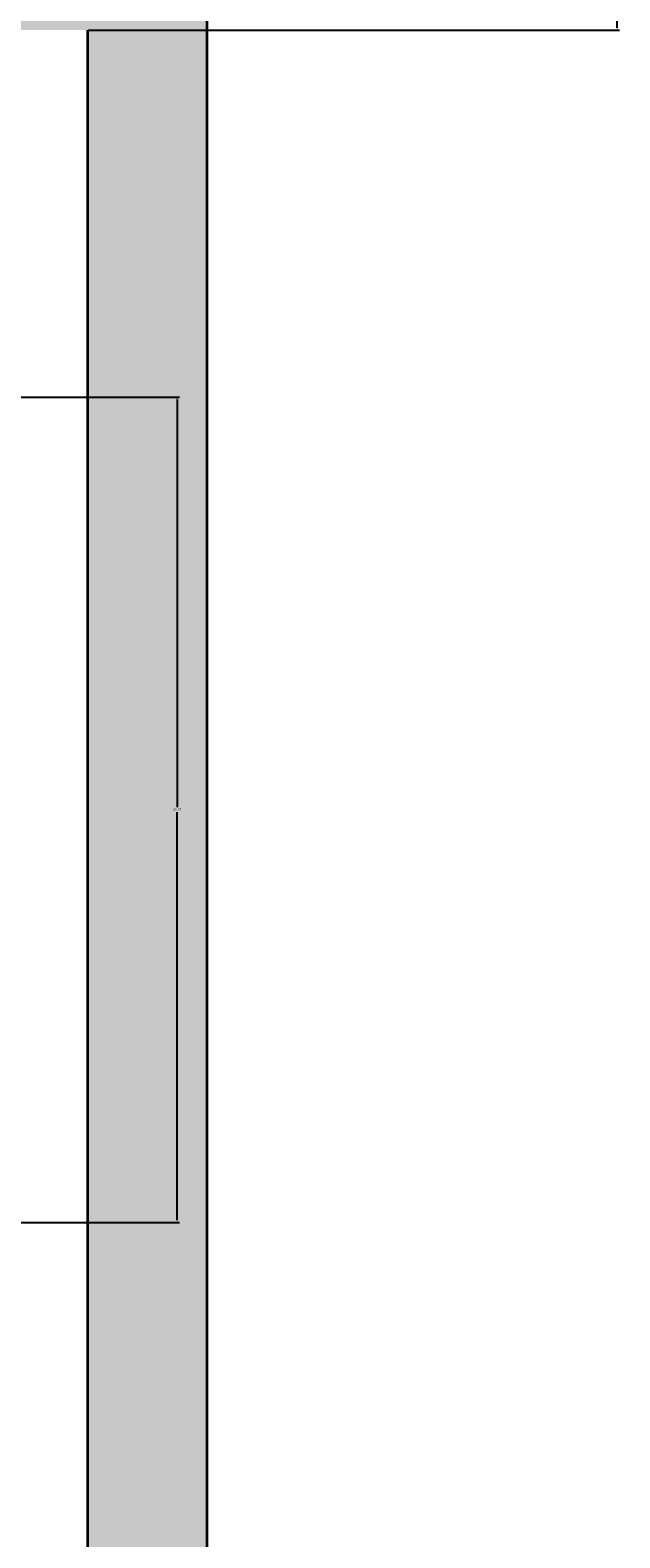
# Model space of a CAD drawing. Units: inches. Extents: x -30 to 437, y -29 to 647.
# Tile 13 of 15: x 392 to 437, y 321 to 435. Entities that reach past the tile are written whole.
import ezdxf

# ---------------------------------------------------------------- set-up
doc = ezdxf.new("R2010")
doc.units = ezdxf.units.IN
doc.header["$MEASUREMENT"] = 0
doc.layers.add('A-ANNO-DIMS', color=2, linetype='Continuous', lineweight=18)
doc.layers.add('A-WALL', color=7, linetype='Continuous', lineweight=35)
doc.layers.add('A-WALL-PATT', color=251, linetype='Continuous', lineweight=13, true_color=0x636466)
doc.styles.get("Standard").update_dxf_attribs({"font": 'arial.ttf'})
doc.dimstyles.get("Standard").update_dxf_attribs({"dimtxt": 0.18, "dimasz": 0.18, "dimexe": 0.18, "dimexo": 0.0625, "dimgap": 0.09, "dimtad": 0, "dimtih": 1, "dimtoh": 1, "dimdec": 4, "dimzin": 0, "dimdsep": 46, "dimtxsty": 'Standard', "dimcen": 0.09, "dimadec": 0, "dimazin": 0, "dimtfac": 1, "dimtdec": 4, "dimtofl": 0, "dimtmove": 0, "dimatfit": 3, "dimfxl": 1, "dimtolj": 1, "dimtzin": 0, "dimarcsym": 0})

# ---------------------------------------------------------------- blocks, each defined once
blk = doc.blocks.new('*D40')
at = {"layer": 'A-ANNO-DIMS', "color": 0, "lineweight": -2, "transparency": 16777216}
for p, q in [((405.74, 615.55), (436.75, 615.55)), ((436.57, 615.37), (436.57, 525.23)), ((436.57, 434.73), (436.57, 524.87)), ((396.74, 434.55), (436.75, 434.55))]:
    blk.add_line(p, q, dxfattribs=at)
at = {"layer": 'A-ANNO-DIMS', "color": 0, "transparency": 16777216}
for points in [[(436.54, 615.37), (436.6, 615.37), (436.57, 615.55)], [(436.54, 434.73), (436.6, 434.73), (436.57, 434.55)]]:
    blk.add_solid(points, dxfattribs=at)
at = {"layer": 'Defpoints', "color": 0, "transparency": 16777216}
for p in [(405.67, 615.55), (436.57, 615.55), (396.67, 434.55)]:
    blk.add_point(p, dxfattribs=at)
at = {"layer": 'A-ANNO-DIMS', "color": 0, "transparency": 16777216, "insert": (436.57, 525.05), "char_height": 0.18, "attachment_point": 5}
blk.add_mtext('\\A1;181', dxfattribs=at)
blk = doc.blocks.new('*D48')
at = {"layer": 'A-ANNO-DIMS', "color": 0, "lineweight": -2, "transparency": 16777216}
for p, q in [((372.59, 406.91), (403.61, 406.91)), ((403.43, 406.73), (403.43, 376.01)), ((403.43, 344.92), (403.43, 375.65)), ((372.59, 344.74), (403.61, 344.74))]:
    blk.add_line(p, q, dxfattribs=at)
at = {"layer": 'A-ANNO-DIMS', "color": 0, "transparency": 16777216}
for points in [[(403.4, 406.73), (403.46, 406.73), (403.43, 406.91)], [(403.4, 344.92), (403.46, 344.92), (403.43, 344.74)]]:
    blk.add_solid(points, dxfattribs=at)
at = {"layer": 'Defpoints', "color": 0, "transparency": 16777216}
for p in [(372.53, 406.91), (372.53, 344.74), (403.43, 344.74)]:
    blk.add_point(p, dxfattribs=at)
at = {"layer": 'A-ANNO-DIMS', "color": 0, "transparency": 16777216, "insert": (403.43, 375.83), "char_height": 0.18, "attachment_point": 5}
blk.add_mtext('\\A1;62.17', dxfattribs=at)

msp = doc.modelspace()

# ---------------------------------------------------------------- hatches: boundary and pattern name
at = {"layer": 'A-WALL-PATT'}
h = msp.add_hatch(color=256, dxfattribs=at)
h.dxf.hatch_style = 1
h.paths.add_polyline_path([(393.6054, 183.2352), (369.6054, 183.2352), (369.6054, 213.2352), (393.6054, 213.2352), (393.6054, 207.2352), (394.6054, 207.2352), (394.6054, 211.2352), (395.6054, 211.2352), (395.6054, 185.2352), (394.6054, 185.2352), (394.6054, 189.2352), (393.6054, 189.2352)], flags=0)
h.paths.add_polyline_path([(384.6054, 189.2352, -1), (390.6054, 189.2352, -1)], flags=0)
h.paths.add_polyline_path([(385.6054, 189.2352, -1), (389.6054, 189.2352, -1)], flags=0)
h.paths.add_polyline_path([(374.6054, 189.2352, -1), (382.6054, 189.2352, -1)], flags=0)
h.paths.add_polyline_path([(386.6054, 189.2352, -1), (388.6054, 189.2352, -1)], flags=0)
h.paths.add_polyline_path([(375.6054, 189.2352, -1), (381.6054, 189.2352, -1)], flags=0)
h.paths.add_polyline_path([(376.6054, 189.2352, -1), (380.6054, 189.2352, -1)], flags=0)
h.paths.add_polyline_path([(377.6054, 189.2352, -1), (379.6054, 189.2352, -1)], flags=0)
h.paths.add_polyline_path([(390.6054, 195.2352), (374.6054, 195.2352), (374.6054, 201.2352), (390.6054, 201.2352)], flags=0)
h.paths.add_polyline_path([(389.6054, 196.2352), (375.6054, 196.2352), (375.6054, 200.2352), (389.6054, 200.2352)], flags=0)
h.paths.add_polyline_path([(383.6054, 207.2352, -1), (391.6054, 207.2352, -1)], flags=0)
h.paths.add_polyline_path([(384.6054, 207.2352, -1), (390.6054, 207.2352, -1)], flags=0)
h.paths.add_polyline_path([(385.6054, 207.2352, -1), (389.6054, 207.2352, -1)], flags=0)
h.paths.add_polyline_path([(386.6054, 207.2352, -1), (388.6054, 207.2352, -1)], flags=0)
h.paths.add_polyline_path([(375.6054, 207.2352, -1), (381.6054, 207.2352, -1)], flags=0)
h.paths.add_polyline_path([(376.6054, 207.2352, -1), (380.6054, 207.2352, -1)], flags=0)
h.paths.add_polyline_path([(377.6054, 207.2352, -1), (379.6054, 207.2352, -1)], flags=0)
h.paths.add_polyline_path([(305.5437, 160.3663, -0.41421356), (304.0437, 158.8663), (271.0437, 158.8663, -0.41421356), (269.5437, 160.3663), (269.5437, 178.3663, -0.41421356), (271.0437, 179.8663), (304.0437, 179.8663, -0.41421356), (305.5437, 178.3663)], flags=0)
h.paths.add_polyline_path([(304.0437, 165.3663, -0.41421356), (303.0437, 164.3663), (289.2937, 164.3663, -0.41421356), (288.2937, 165.3663), (288.2937, 177.3663, -0.41421356), (289.2937, 178.3663), (303.0437, 178.3663, -0.41421356), (304.0437, 177.3663)], flags=0)
h.paths.add_polyline_path([(296.5437, 171.3663, -1), (295.5437, 171.3663, -1)], flags=0)
h.paths.add_polyline_path([(286.7937, 165.3663, -0.41421356), (285.7937, 164.3663), (272.0437, 164.3663, -0.41421356), (271.0437, 165.3663), (271.0437, 177.3663, -0.41421356), (272.0437, 178.3663), (285.7937, 178.3663, -0.41421356), (286.7937, 177.3663)], flags=0)
h.paths.add_polyline_path([(279.5437, 171.3663, -1), (278.5437, 171.3663, -1)], flags=0)
h.paths.add_polyline_path([(360.6737, 290.5474), (360.6737, 300.5474), (396.6737, 300.5474), (396.6737, 290.5474)], flags=0)
h.paths.add_polyline_path([(259.6737, 124.5474), (259.6737, 114.5474), (171.6737, 114.5474), (171.6737, 124.5474)], flags=0)
h.paths.add_polyline_path([(288.0737, 215.3705), (286.7097, 214.583), (268.7097, 245.7599), (270.0737, 246.5474)], flags=0)
h.paths.add_polyline_path([(259.6737, 168.5474), (256.6737, 168.5474), (256.6737, 173.5474), (256.6737, 179.0224), (255.8753, 177.6395), (224.2956, 195.872, 0.12053744), (220.1737, 179.0224, 0.12053744), (216.0518, 195.872), (184.4721, 177.6395), (183.6737, 179.0224), (215.2836, 197.2724), (216.0821, 195.8895), (216.0518, 195.872, -0.12053744), (220.1737, 179.0224, -0.12053744), (224.2956, 195.872), (224.2653, 195.8895), (225.0638, 197.2724), (256.6737, 179.0224), (256.6737, 173.5474), (259.6737, 173.5474)], flags=0)
h.paths.add_polyline_path([(386.7943, 325.4601), (372.6871, 325.4601), (372.6871, 339.5673), (386.7943, 339.5673)], flags=0)
h.paths.add_polyline_path([(359.5875, 343.7429), (357.7905, 343.7429), (357.7905, 327.9179), (359.3933, 327.9179, 0.41420885), (361.5302, 330.0549), (361.5302, 341.8434, 0.41436161)], flags=0)
h.paths.add_polyline_path([(341.7887, 323.1235, -0.11921667), (340.7839, 323.1235)], flags=0)
h.paths.add_polyline_path([(379.6332, 328.8632), (379.6332, 332.2699), (376.0992, 332.2699, 0.39427733)], flags=0)
h.paths.add_polyline_path([(375.5299, 332.459, -1), (383.8511, 332.459, -1)], flags=0)
h.paths.add_polyline_path([(388.9363, 344.7425), (372.5309, 344.7425, -0.41421356), (370.394, 346.8794), (370.394, 347.5594, -0.39085173), (372.3472, 349.7005, -0.43951011), (370.394, 351.4933), (370.394, 365.1894, -0.40305452), (372.2191, 367.1298, -0.41839453), (370.394, 368.9291), (370.394, 382.6251, -0.40885826), (372.2519, 384.5722, -0.42377324), (370.394, 386.3707), (370.394, 400.0667, -0.38660687), (372.1327, 402.0094), (372.531, 402.0094, -0.41421834), (370.394, 404.1464), (370.394, 404.7778, -0.41420891), (372.5309, 406.9147), (388.9363, 406.9147, -0.41421821), (391.0733, 404.7778), (391.0733, 346.8794, -0.41421356)], flags=0)
edge = h.paths.add_edge_path(flags=0)
edge.add_spline(control_points=[(349.3585, 363.204), (349.0859, 363.204), (348.8133, 363.2227), (348.2712, 363.2973), (348.0016, 363.3531), (347.3533, 363.5328), (346.9776, 363.6755), (346.2445, 364.0308), (345.887, 364.2432), (345.1953, 364.7329), (344.8611, 365.0101), (344.2197, 365.6237), (343.9125, 365.9603), (343.211, 366.8336), (342.8313, 367.3965), (342.1401, 368.6117), (341.8286, 369.2641), (341.2807, 370.64), (341.0443, 371.3636), (340.6522, 372.8619), (340.4964, 373.6367), (340.2695, 375.2158), (340.1983, 376.0203), (340.142, 377.6365), (340.157, 378.4483), (340.2729, 380.0567), (340.3738, 380.8533), (340.6589, 382.4093), (340.8432, 383.1686), (341.2906, 384.629), (341.5538, 385.3301), (342.1531, 386.6544), (342.4891, 387.2776), (343.2266, 388.4288), (343.6281, 388.9567), (344.4879, 389.9012), (344.9463, 390.3178), (345.7981, 390.9428), (346.182, 391.1771), (346.9712, 391.5648), (347.3766, 391.7182), (348.2004, 391.9387), (348.6189, 392.0058), (349.4588, 392.0508), (349.8801, 392.0288), (350.7146, 391.8966), (351.1278, 391.7865), (351.9366, 391.4822), (352.3323, 391.2882), (353.0989, 390.8223), (353.4699, 390.5504), (354.1819, 389.9355), (354.5229, 389.5924), (355.1706, 388.8418), (355.4772, 388.4343), (356.1315, 387.4422), (356.4671, 386.8397), (357.0692, 385.5581), (357.3356, 384.879), (357.7933, 383.4624), (357.9846, 382.725), (358.2875, 381.2112), (358.3992, 380.4349), (358.5404, 378.8643), (358.5699, 378.0699), (358.546, 376.4841), (358.4926, 375.6928), (358.3042, 374.1343), (358.1692, 373.3672), (357.8207, 371.8774), (357.6072, 371.1549), (357.1067, 369.7735), (356.8196, 369.1148), (356.1782, 367.8787), (355.8238, 367.3013), (355.0551, 366.244), (354.6408, 365.7641), (353.7607, 364.9161), (353.2948, 364.5481), (352.445, 364.0149), (352.0701, 363.822), (351.3034, 363.5117), (350.9116, 363.3943), (350.1325, 363.2418), (349.7455, 363.204), (349.3585, 363.204)], knot_values=[3.14159265, 3.14159265, 3.14159265, 3.14159265, 3.22691715, 3.22691715, 3.31224165, 3.31224165, 3.43426671, 3.43426671, 3.55629177, 3.55629177, 3.67831683, 3.67831683, 3.8003419, 3.8003419, 3.97157384, 3.97157384, 4.14280577, 4.14280577, 4.31403771, 4.31403771, 4.48526965, 4.48526965, 4.65650159, 4.65650159, 4.82773353, 4.82773353, 4.99896547, 4.99896547, 5.1701974, 5.1701974, 5.34142934, 5.34142934, 5.51266128, 5.51266128, 5.68389322, 5.68389322, 5.85512516, 5.85512516, 5.98669107, 5.98669107, 6.11825699, 6.11825699, 6.24982291, 6.24982291, 6.38138882, 6.38138882, 6.51295474, 6.51295474, 6.64452065, 6.64452065, 6.77608657, 6.77608657, 6.90765249, 6.90765249, 7.0392184, 7.0392184, 7.20701563, 7.20701563, 7.37481286, 7.37481286, 7.54261009, 7.54261009, 7.71040732, 7.71040732, 7.87820455, 7.87820455, 8.04600178, 8.04600178, 8.21379901, 8.21379901, 8.38159624, 8.38159624, 8.54939347, 8.54939347, 8.7171907, 8.7171907, 8.88498794, 8.88498794, 9.05278517, 9.05278517, 9.17820699, 9.17820699, 9.30362881, 9.30362881, 9.42477796, 9.42477796, 9.42477796, 9.42477796], degree=3, periodic=0)
edge.add_line((341.1696, 384.3006), (341.2012, 384.2808))
edge = h.paths.add_edge_path(flags=0)
edge.add_line((344.3353, 388.7801), (344.317, 388.7915))
edge.add_ellipse((349.3585, 377.6204), major_axis=(0, -13.7895), ratio=0.62186025, start_angle=-244.867444, end_angle=-124.769923)
h.paths.add_polyline_path([(163.6737, 163.1474), (132.4968, 145.1474), (131.7093, 146.5114), (162.8862, 164.5114)], flags=0)
h.paths.add_polyline_path([(366.4355, 409.0896, -0.41423669), (364.2985, 406.9525, -0.4913499), (361.5302, 408.8973), (361.5302, 420.6405, 0.41421356), (359.3932, 422.7775), (357.7905, 422.7775), (357.7905, 406.9525), (359.6317, 406.9525, 0.42741026), (361.5332, 408.9757, 0.39869469), (363.6672, 406.9525, 0.51958103), (366.4355, 409.0895)], flags=0)
h.paths.add_polyline_path([(386.7943, 410.9671), (372.6871, 410.9671), (372.6871, 425.0742), (386.7943, 425.0742)], flags=0)
h.paths.add_polyline_path([(379.6332, 414.3701), (379.6332, 417.7768), (376.0992, 417.7768, 0.39427733)], flags=0)
h.paths.add_polyline_path([(375.5299, 417.966, -1), (383.8511, 417.966, -1)], flags=0)
h.paths.add_polyline_path([(150.0377, 351.583), (148.6737, 352.3705), (166.6737, 383.5474), (168.0377, 382.7599)], flags=0)
h.paths.add_polyline_path([(91.6737, 234.1974), (66.559, 219.6974), (65.9246, 220.7962), (91.0393, 235.2962)], flags=0)
h.paths.add_polyline_path([(255.4612, 443.5834), (254.6737, 444.9474), (285.8506, 462.9474), (286.6381, 461.5834)], flags=0)
h.paths.add_polyline_path([(176.2737, 394.5474), (158.2737, 425.7243), (159.6377, 426.5118), (177.6377, 395.3349)], flags=0)
h.paths.add_polyline_path([(243.6737, 439.5474), (243.0393, 438.4486), (217.9246, 452.9486), (218.559, 454.0474)], flags=0)
h.paths.add_polyline_path([(38.1264, 269.8429), (40.2408, 269.8429), (40.2408, 270.3508), (38.1264, 270.3508)], flags=0)
h.paths.add_polyline_path([(75.7157, 289.9439), (40.2408, 289.9439), (38.1264, 289.6524), (40.2408, 289.6524)], flags=0)
h.paths.add_polyline_path([(75.7157, 270.0846), (77.6447, 270.0846), (77.6697, 270.1626), (75.7175, 270.1626)], flags=0)
h.paths.add_polyline_path([(80.5373, 293.3002), (33.0467, 293.3002), (13.5054, 293.3002), (13.5054, 351.9244), (29.7898, 351.9244), (80.5373, 351.9244)], flags=0)
h.paths.add_polyline_path([(46.0261, 212.466, -0.50131678), (27.1651, 207.5106), (21.165, 209.5107), (21.165, 206.5107), (22.665, 206.5107), (22.665, 203.5107), (21.165, 203.5107), (21.165, 203.0107), (13.165, 203.0107), (13.165, 224.0107), (21.165, 224.0107), (21.165, 217.5107), (27.1649, 219.5106, -0.50132349), (46.0261, 214.5554, -0.13289091)], flags=0)
h.paths.add_polyline_path([(44.688, 211.8666, -0.48007965), (27.165, 209.5107), (27.165, 217.5107, -0.4800795), (44.688, 215.1547, -0.21500378)], flags=0)
h.paths.add_polyline_path([(19.415, 204.0107), (15.165, 204.0107, -0.41421356), (14.165, 204.7607), (14.165, 222.0107, -0.41421356), (14.915, 223.0107), (19.165, 223.0107, -0.41421356), (20.165, 222.2607), (20.165, 205.0107, -0.41421356)], flags=0)
h.paths.add_polyline_path([(32.7608, 269.0719), (31.8439, 269.0719), (31.8439, 268.6134), (13.5054, 268.6134), (13.5054, 291.5366), (31.8439, 291.5366), (32.7608, 291.0781), (32.7608, 280.9919, -1), (32.7608, 279.1581)], flags=0)
h.paths.add_polyline_path([(40.2408, 360.1436), (38.1264, 360.1436), (38.1264, 359.6357), (40.2408, 359.6357)], flags=0)
h.paths.add_polyline_path([(75.7157, 355.2807), (40.2408, 355.2807), (38.1264, 355.5722), (40.2408, 355.5722), (40.2408, 355.2807), (75.7157, 355.2807), (75.7157, 375.5982), (40.2408, 375.5982), (38.1264, 375.3817), (40.2408, 375.3817), (40.2408, 375.5982), (75.7157, 375.5982), (77.9733, 375.062), (75.7175, 375.062), (75.7175, 374.554)], flags=0)
h.paths.add_polyline_path([(42.8174, 299.814, 0.13867074), (34.1602, 294.603), (14.8081, 294.603), (14.8081, 350.6216), (29.8539, 350.6216, 0.09822056)], flags=0)
h.paths.add_polyline_path([(15.8636, 276.7781, -0.30640166), (20.3757, 283.4499), (20.3483, 290.6726), (31.4014, 290.7146), (31.4309, 282.9124), (26.8287, 282.895, -0.26006276), (30.241, 276.7781, -1)], flags=0)
h.paths.add_polyline_path([(26.1332, 276.7781), (23.0523, 273.6972), (19.9714, 276.7781), (23.0523, 279.8589), (23.0523, 283.9209), (21.3493, 283.9145), (20.7006, 283.5219), (20.6907, 286.1226), (23.2914, 286.1325), (25.8936, 285.7522), (27.1939, 285.7572), (28.4928, 286.1522), (31.0935, 286.1621), (31.0918, 286.6172), (25.6303, 286.5965), (25.616, 290.3675), (31.0775, 290.3882), (31.0918, 286.6172), (31.1034, 283.5614), (28.5027, 283.5515), (25.9005, 283.9317), (23.0523, 283.9209), (23.0523, 279.8589)], flags=0)
h.paths.add_polyline_path([(24.0793, 276.7781, -1), (22.0253, 276.7781, -1)], flags=0)
h.paths.add_polyline_path([(35.7687, 302.2895, -0.41421356), (35.2283, 301.2726), (22.2164, 297.2909, -0.41421356), (21.1995, 297.8313), (15.7317, 315.6996, -0.41421356), (16.2721, 316.7165), (18.8554, 317.507), (15.3721, 328.8904, -0.41421356), (15.9125, 329.9073), (28.9244, 333.889, -0.41421356), (29.9414, 333.3486), (35.4091, 315.4802, -0.41421356), (34.8687, 314.4633), (32.2854, 313.6728)], flags=0)
h.paths.add_polyline_path([(361.3728, 532.6207), (302.7487, 532.6207), (302.7487, 580.1113), (302.7487, 599.6527), (361.3728, 599.6527), (361.3728, 583.3682)], flags=0)
h.paths.add_polyline_path([(370.1, 575.0316), (370.1, 572.9172), (370.6079, 572.9172), (370.6079, 575.0316)], flags=0)
h.paths.add_polyline_path([(385.0466, 537.4423), (385.0466, 572.9172), (384.8302, 575.0316), (384.8302, 572.9172)], flags=0)
h.paths.add_polyline_path([(384.5104, 535.3262), (384.5104, 537.4406), (384.0025, 537.4406), (364.7291, 537.4423), (364.7291, 572.9172), (365.0206, 575.0316), (365.0206, 572.9172), (364.7291, 572.9172), (364.7291, 537.4423), (384.5884, 537.4423), (384.5884, 535.5133)], flags=0)
h.paths.add_polyline_path([(384.5884, 535.5133), (383.4945, 535.164), (383.4945, 537.4406), (382.9866, 535.3262), (382.9866, 537.4406), (383.4945, 535.3262), (383.4945, 537.4406), (384.5884, 537.4406)], flags=0)
h.paths.add_polyline_path([(23.874, 286.8174), (21.0132, 286.8065), (21.0004, 290.1875), (23.8612, 290.1983)], flags=0)
h.paths.add_polyline_path([(242.9824, 511.1667), (234.9824, 511.1667), (234.9824, 517.6667), (228.9825, 515.6667, -0.50132349), (210.1213, 520.622, -0.13289091), (210.1213, 522.7114, -0.50131678), (228.9823, 527.6667), (234.9824, 525.6667), (234.9824, 528.6667), (233.4824, 528.6667), (233.4824, 531.6667), (234.9824, 531.6667), (234.9824, 532.1667), (242.9824, 532.1667)], flags=0)
h.paths.add_polyline_path([(236.9824, 512.1667, -0.41421356), (235.9824, 512.9167), (235.9824, 530.1667, -0.41421356), (236.7324, 531.1667), (240.9824, 531.1667, -0.41421356), (241.9824, 530.4167), (241.9824, 513.1667, -0.41421356), (241.2324, 512.1667)], flags=0)
h.paths.add_polyline_path([(279.533, 537.4423), (279.533, 535.5133), (279.6111, 535.4884), (279.6111, 537.4406)], flags=0)
h.paths.add_polyline_path([(279.2913, 575.0316), (279.2913, 572.9172), (279.7992, 572.9172), (279.7992, 575.0316)], flags=0)
h.paths.add_polyline_path([(211.4594, 520.0227, -0.21500378), (211.4594, 523.3107, -0.48007965), (228.9824, 525.6667), (228.9824, 517.6667, -0.4800795)], flags=0)
h.paths.add_polyline_path([(32.7627, 354.1465), (31.8457, 354.1465), (31.8457, 353.688), (13.5054, 353.688), (13.5054, 376.6134), (31.8457, 376.6134), (32.7627, 376.1549), (32.7627, 366.0677, -1), (32.7627, 364.2337)], flags=0)
h.paths.add_polyline_path([(15.9446, 365.1507, -1), (30.3234, 365.1507, -1)], flags=0)
h.paths.add_polyline_path([(41.213, 428.467), (43.3274, 428.467), (43.3274, 428.9749), (41.213, 428.9749)], flags=0)
h.paths.add_polyline_path([(78.8022, 448.568), (43.3274, 448.568), (41.213, 448.2765), (43.3274, 448.2765)], flags=0)
h.paths.add_polyline_path([(78.8022, 428.7087), (80.7313, 428.7087), (80.7562, 428.7868), (78.804, 428.7868)], flags=0)
h.paths.add_polyline_path([(26.2152, 365.1507), (23.134, 362.0696), (20.0529, 365.1507), (23.134, 368.2319)], flags=0)
h.paths.add_polyline_path([(24.1611, 365.1507, -1), (22.107, 365.1507, -1)], flags=0)
h.paths.add_polyline_path([(309.2625, 570.3406, 0.13867074), (304.0514, 578.9978), (304.0514, 598.3499), (360.07, 598.3499), (360.07, 583.3041, 0.09822056)], flags=0)
h.paths.add_polyline_path([(246.6737, 552.5474), (129.6737, 552.5474), (129.6737, 606.5474), (246.6737, 606.5474)], flags=16)
h.paths.add_polyline_path([(373.6822, 580.3953), (363.595, 580.3953), (363.595, 581.3123), (363.1365, 581.3123), (363.1365, 599.6527), (386.0619, 599.6527), (386.0619, 581.3123), (385.6034, 580.3953), (375.5162, 580.3953, -1)], flags=0)
h.paths.add_polyline_path([(83.6239, 451.9244), (36.1333, 451.9244), (16.5919, 451.9244), (16.5919, 510.5485), (32.8764, 510.5485), (83.6239, 510.5485)], flags=0)
h.paths.add_polyline_path([(367.4098, 590.024, -1), (381.7886, 590.024, -1)], flags=0)
h.paths.add_polyline_path([(374.5992, 586.9428), (371.518, 590.024), (374.5992, 593.1052), (377.6803, 590.024)], flags=0)
h.paths.add_polyline_path([(373.5721, 590.024, -1), (375.6262, 590.024, -1)], flags=0)
h.paths.add_polyline_path([(324.9287, 577.7489, -0.41421356), (323.9118, 578.2893), (323.1212, 580.8726), (311.7379, 577.3893, -0.41421356), (310.721, 577.9297), (306.7393, 590.9416, -0.41421356), (307.2797, 591.9585), (325.1481, 597.4263, -0.41421356), (326.165, 596.8859), (326.9555, 594.3026), (338.3388, 597.7859, -0.41421356), (339.3557, 597.2455), (343.3374, 584.2336, -0.41421356), (342.797, 583.2167)], flags=0)
h.paths.add_polyline_path([(300.5265, 580.3972), (290.4404, 580.3972, -1), (288.6065, 580.3972), (278.5203, 580.3972), (278.5203, 581.3142), (278.0619, 581.3142), (278.0619, 599.6527), (300.985, 599.6527), (300.985, 581.3142)], flags=0)
h.paths.add_polyline_path([(300.163, 581.7567), (292.3609, 581.7271), (292.3434, 586.3294, -0.75567924), (279.0378, 590.1057, -0.82536731), (292.8983, 592.7823), (300.1211, 592.8097)], flags=0)
h.paths.add_polyline_path([(299.8367, 582.0805), (296.0656, 582.0662), (293.0098, 582.0546), (292.9999, 584.6553), (293.3802, 587.2575), (293.3694, 590.1057), (289.3074, 590.1057), (286.2265, 587.0248), (283.1456, 590.1057), (286.2265, 593.1866), (289.3074, 590.1057), (293.3694, 590.1057), (293.3629, 591.8088), (292.9703, 592.4575), (295.5711, 592.4673), (295.5809, 589.8666), (295.2007, 587.2644), (295.2056, 585.9641), (295.6006, 584.6652), (295.6105, 582.0645), (296.0656, 582.0662), (296.0449, 587.5277), (299.8159, 587.542)], flags=0)
h.paths.add_polyline_path([(285.1995, 590.1057, -1), (287.2535, 590.1057, -1)], flags=0)
h.paths.add_polyline_path([(299.6467, 589.2969), (296.2658, 589.284), (296.255, 592.1448), (299.6359, 592.1576)], flags=0)
h.paths.add_polyline_path([(35.8473, 427.696), (34.9304, 427.696), (34.9304, 427.2376), (16.5919, 427.2376), (16.5919, 450.1607), (34.9304, 450.1607), (35.8473, 449.7022), (35.8473, 439.6161, -1), (35.8473, 437.7822)], flags=0)
h.paths.add_polyline_path([(18.9502, 435.4022, -0.30640166), (23.4623, 442.074), (23.4349, 449.2968), (34.4879, 449.3387), (34.5175, 441.5366), (29.9152, 441.5191, -0.26006276), (33.3275, 435.4022, -1)], flags=0)
h.paths.add_polyline_path([(29.2197, 435.4022), (26.1389, 432.3213), (23.058, 435.4022), (26.1389, 438.4831), (26.1389, 442.5451), (24.4358, 442.5386), (23.7871, 442.1461), (23.7772, 444.7468), (26.378, 444.7566), (28.9801, 444.3764), (30.2805, 444.3813), (31.5794, 444.7764), (34.1801, 444.7862), (34.1784, 445.2413), (28.7169, 445.2206), (28.7026, 448.9917), (34.164, 449.0124), (34.1784, 445.2413), (34.1899, 442.1855), (31.5892, 442.1756), (28.987, 442.5559), (26.1389, 442.5451), (26.1389, 438.4831)], flags=0)
h.paths.add_polyline_path([(27.1658, 435.4022, -1), (25.1119, 435.4022, -1)], flags=0)
h.paths.add_polyline_path([(45.904, 458.4382, 0.13867074), (37.2467, 453.2271), (17.8947, 453.2271), (17.8947, 509.2457), (32.9405, 509.2457, 0.09822056)], flags=0)
h.paths.add_polyline_path([(26.9605, 445.4415), (24.0997, 445.4307), (24.0869, 448.8116), (26.9477, 448.8225)], flags=0)
h.paths.add_polyline_path([(38.3149, 459.8967), (25.3029, 455.915, -0.41421356), (24.286, 456.4554), (18.8183, 474.3238, -0.41421356), (19.3586, 475.3407), (21.942, 476.1312), (18.4587, 487.5145, -0.41421356), (18.999, 488.5314), (32.011, 492.5131, -0.41421356), (33.0279, 491.9727), (38.4957, 474.1044, -0.41421356), (37.9553, 473.0875), (35.3719, 472.297), (38.8553, 460.9136, -0.41421356)], flags=0)
h.paths.add_polyline_path([(43.3274, 518.7678), (41.213, 518.7678), (41.213, 518.2598), (43.3274, 518.2598)], flags=0)
h.paths.add_polyline_path([(78.8022, 513.9049), (43.3274, 513.9049), (41.213, 514.1964), (43.3274, 514.1964), (43.3274, 513.9049), (78.8022, 513.9049), (78.8022, 534.2223), (43.3274, 534.2223), (41.213, 534.0059), (43.3274, 534.0059), (43.3274, 534.2223), (78.8022, 534.2223), (81.0599, 533.6861), (78.804, 533.6861), (78.804, 533.1782)], flags=0)
h.paths.add_polyline_path([(121.6737, 556.8974), (121.0393, 555.7986), (95.9246, 570.2986), (96.559, 571.3974)], flags=0)
h.paths.add_polyline_path([(35.8493, 512.7707), (34.9322, 512.7707), (34.9322, 512.3122), (16.5919, 512.3122), (16.5919, 535.2376), (34.9322, 535.2376), (35.8493, 534.7791), (35.8493, 524.6919, -1), (35.8493, 522.8579)], flags=0)
h.paths.add_polyline_path([(19.0312, 523.7749, -1), (33.41, 523.7749, -1)], flags=0)
h.paths.add_polyline_path([(26.2206, 520.6937), (23.1394, 523.7749), (26.2206, 526.8561), (29.3018, 523.7749)], flags=0)
h.paths.add_polyline_path([(25.1935, 523.7749, -1), (27.2476, 523.7749, -1)], flags=0)
h.paths.add_polyline_path([(28.4381, 586.0173), (22.438, 588.0173), (22.438, 585.0173), (23.938, 585.0173), (23.938, 582.0173), (22.438, 582.0173), (22.438, 581.5173), (14.438, 581.5173), (14.438, 602.5173), (22.438, 602.5173), (22.438, 596.0173), (28.4379, 598.0173, -0.50132349), (47.2992, 593.062, -0.13289091), (47.2992, 590.9726, -0.50131678)], flags=0)
h.paths.add_polyline_path([(28.438, 588.0174), (28.438, 596.0173, -0.4800795), (45.961, 593.6614, -0.21500378), (45.961, 590.3733, -0.48007965)], flags=0)
h.paths.add_polyline_path([(20.688, 582.5173), (16.438, 582.5173, -0.41421356), (15.438, 583.2673), (15.438, 600.5173, -0.41421356), (16.188, 601.5173), (20.438, 601.5173, -0.41421356), (21.438, 600.7673), (21.438, 583.5173, -0.41421356)], flags=0)
h.paths.add_polyline_path([(171.6737, 2.0474), (171.6737, 104.5474), (259.6737, 104.5474), (259.6737, 148.5474), (396.6737, 148.5474), (396.6737, 2.0474), (405.6737, 2.0474), (405.6737, 615.5474), (1.6737, 615.5474), (1.6737, 2.0474)])
h.paths.add_polyline_path([(171.6737, 104.5474), (259.6737, 104.5474), (259.6737, 210.5474), (264.6737, 210.5474), (264.6737, 153.5474), (396.6737, 153.5474), (396.6737, 249.5474), (264.6737, 249.5474), (264.6737, 246.5474), (259.6737, 246.5474), (259.6737, 254.5474), (396.6737, 254.5474), (396.6737, 434.5474), (290.6737, 434.5474), (290.6737, 439.5474), (396.6737, 439.5474), (396.6737, 606.5474), (251.6737, 606.5474), (251.6737, 439.5474), (254.6737, 439.5474), (254.6737, 434.5474), (243.6737, 434.5474), (243.6737, 439.5474), (246.6737, 439.5474), (246.6737, 547.5474), (186.6737, 547.5474), (186.6737, 439.5474), (214.6737, 439.5474), (214.6737, 434.5474), (186.6737, 434.5474), (186.6737, 430.5474), (181.6737, 430.5474), (181.6737, 547.5474), (121.6737, 547.5474), (121.6737, 552.5474), (124.6737, 552.5474), (124.6737, 606.5474), (10.6737, 606.5474), (10.6737, 552.5474), (92.6737, 552.5474), (92.6737, 547.5474), (10.6737, 547.5474), (10.6737, 391.5474), (181.6737, 391.5474), (181.6737, 394.5474), (186.6737, 394.5474), (186.6737, 386.5474), (171.6737, 386.5474), (171.6737, 383.5474), (166.6737, 383.5474), (166.6737, 386.5474), (10.6737, 386.5474), (10.6737, 238.5474), (62.6737, 238.5474), (62.6737, 233.5474), (10.6737, 233.5474), (10.6737, 173.5474), (94.6737, 173.5474), (94.6737, 233.5474), (91.6737, 233.5474), (91.6737, 238.5474), (166.6737, 238.5474), (166.6737, 347.5474), (171.6737, 347.5474), (171.6737, 233.5474), (99.6737, 233.5474), (99.6737, 173.5474), (127.6737, 173.5474), (127.6737, 168.5474), (10.6737, 168.5474), (10.6737, 11.0474), (166.6737, 11.0474), (166.6737, 168.5474), (163.6737, 168.5474), (163.6737, 173.5474), (183.6737, 173.5474), (183.6737, 168.5474), (171.6737, 168.5474)])

# ---------------------------------------------------------------- linework, layer by layer
at = {"layer": 'A-WALL'}
msp.add_line((396.6737, 434.5474), (396.6737, 254.5474), dxfattribs=at)
msp.add_lwpolyline([(171.6737, 2.0474), (1.6737, 2.0474), (1.6737, 615.5474), (405.6737, 615.5474), (405.6737, 2.0474), (396.6737, 2.0474)], dxfattribs=at)

# ---------------------------------------------------------------- dimensions: what is measured, and where the dimension line sits
at = {"layer": 'A-ANNO-DIMS'}
for base, p1, p2, angle, override, picture, middle in [((436.5737, 615.5474), (396.6737, 434.5474), (405.6737, 615.5474), 90, {"dimdec": 0, "dimlfac": 1, "dimrnd": 0, "dimzin": 0, "dimdsep": 46, "dimlunit": 2}, '*D40', (436.5737, 525.0474)), ((403.4309, 344.7425), (372.5309, 406.9147), (372.5309, 344.7425), 270, {"dimdec": 2, "dimlfac": 1, "dimrnd": 0, "dimzin": 0, "dimdsep": 46, "dimlunit": 2}, '*D48', (403.4309, 375.8286))]:
    dim = msp.add_linear_dim(base=base, p1=p1, p2=p2, angle=angle, dimstyle='Standard', override=override, dxfattribs=at)
    dim.commit()
    dim.dimension.update_dxf_attribs({"geometry": picture, "text_midpoint": middle})

doc.saveas('drawing.dxf')
